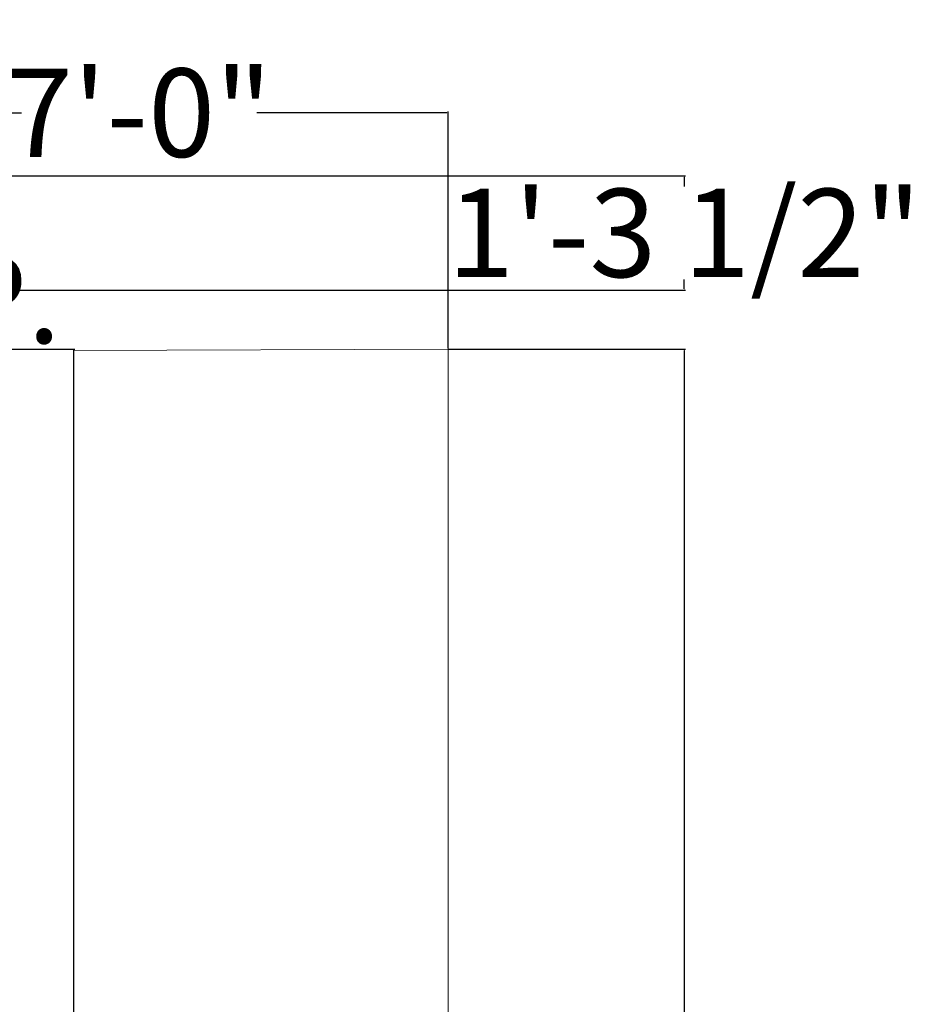
# Model space of a CAD drawing. Units: inches. Extents: x 1063 to 2718, y 423 to 1923.
# Tile 7 of 7: x 1509 to 1630, y 862 to 996. Entities that reach past the tile are written whole.
import ezdxf

# ---------------------------------------------------------------- set-up
doc = ezdxf.new("R2010")
doc.units = ezdxf.units.IN
doc.header["$LTSCALE"] = 6
doc.header["$MEASUREMENT"] = 0
doc.layers.add('A-ANNO-DIMS', color=2, linetype='Continuous', lineweight=18)
doc.layers.add('C-PKNG', color=7, linetype='Continuous', lineweight=18)
doc.styles.get("Standard").update_dxf_attribs({"font": 'arial.ttf'})
doc.dimstyles.get("Standard").update_dxf_attribs({"dimtxt": 12, "dimasz": 0.18, "dimexe": 0.18, "dimexo": 0.0625, "dimgap": 0.09, "dimtad": 0, "dimtih": 1, "dimtoh": 1, "dimdec": 1, "dimzin": 0, "dimdsep": 46, "dimlunit": 3, "dimtxsty": 'Standard', "dimcen": 0.09, "dimadec": 0, "dimazin": 0, "dimtfac": 1, "dimtdec": 1, "dimtofl": 0, "dimtmove": 0, "dimatfit": 3, "dimfxl": 1, "dimtolj": 1, "dimtzin": 0, "dimarcsym": 0})

# ---------------------------------------------------------------- blocks, each defined once
blk = doc.blocks.new('*D3')
at = {"layer": 'A-ANNO-DIMS', "color": 0, "lineweight": -2, "ltscale": 6, "transparency": 16777216}
for p, q in [((1482.99, 951.12), (1516.18, 951.12)), ((1516, 950.94), (1516, 765.34)), ((1516, 567.3), (1516, 752.9)), ((1482.99, 567.12), (1516.18, 567.12))]:
    blk.add_line(p, q, dxfattribs=at)
at = {"layer": 'A-ANNO-DIMS', "color": 0, "ltscale": 6, "transparency": 16777216}
for points in [[(1515.97, 950.94), (1516.03, 950.94), (1516, 951.12)], [(1515.97, 567.3), (1516.03, 567.3), (1516, 567.12)]]:
    blk.add_solid(points, dxfattribs=at)
at = {"layer": 'Defpoints', "color": 0, "ltscale": 6, "transparency": 16777216}
for p in [(1482.93, 951.12), (1516, 951.12), (1482.93, 567.12)]:
    blk.add_point(p, dxfattribs=at)
at = {"layer": 'A-ANNO-DIMS', "color": 0, "ltscale": 6, "transparency": 16777216, "insert": (1516, 759.12), "char_height": 12, "attachment_point": 5}
blk.add_mtext("\\A1;32'", dxfattribs=at)
blk = doc.blocks.new('*D36')
at = {"layer": 'A-ANNO-DIMS', "color": 0, "lineweight": -2, "ltscale": 6, "transparency": 16777216}
for p, q in [((1334.27, 958.87), (1334.27, 957.74)), ((1334.45, 957.92), (1340.83, 957.92)), ((1341.01, 958.87), (1341.01, 957.74)), ((1341.01, 957.92), (1341.19, 957.92))]:
    blk.add_line(p, q, dxfattribs=at)
at = {"layer": 'A-ANNO-DIMS', "color": 0, "ltscale": 6, "transparency": 16777216}
for points in [[(1334.45, 957.95), (1334.45, 957.89), (1334.27, 957.92)], [(1340.83, 957.95), (1340.83, 957.89), (1341.01, 957.92)]]:
    blk.add_solid(points, dxfattribs=at)
at = {"layer": 'Defpoints', "color": 0, "ltscale": 6, "transparency": 16777216}
for p in [(1334.27, 958.93), (1341.01, 958.93), (1341.01, 957.92)]:
    blk.add_point(p, dxfattribs=at)
at = {"layer": 'A-ANNO-DIMS', "color": 0, "ltscale": 6, "transparency": 16777216, "insert": (1429.29, 957.92), "char_height": 12, "attachment_point": 5}
blk.add_mtext('\\A1;BURNER 0\'-6 1/2" TYP.', dxfattribs=at)
blk = doc.blocks.new('*D48')
at = {"layer": 'A-ANNO-DIMS', "color": 0, "lineweight": -2, "ltscale": 6, "transparency": 16777216}
for p, q in [((1482.93, 951.18), (1482.93, 983.4)), ((1483.11, 983.22), (1508.94, 983.22)), ((1566.75, 983.22), (1540.92, 983.22)), ((1566.93, 951.18), (1566.93, 983.4))]:
    blk.add_line(p, q, dxfattribs=at)
at = {"layer": 'A-ANNO-DIMS', "color": 0, "ltscale": 6, "transparency": 16777216}
for points in [[(1483.11, 983.25), (1483.11, 983.19), (1482.93, 983.22)], [(1566.75, 983.25), (1566.75, 983.19), (1566.93, 983.22)]]:
    blk.add_solid(points, dxfattribs=at)
at = {"layer": 'Defpoints', "color": 0, "ltscale": 6, "transparency": 16777216}
for p in [(1566.93, 983.22), (1482.93, 951.12), (1566.93, 951.12)]:
    blk.add_point(p, dxfattribs=at)
at = {"layer": 'A-ANNO-DIMS', "color": 0, "ltscale": 6, "transparency": 16777216, "insert": (1524.93, 983.22), "char_height": 12, "attachment_point": 5}
blk.add_mtext('\\A1;7\'-0"', dxfattribs=at)
blk = doc.blocks.new('*D49')
at = {"layer": 'A-ANNO-DIMS', "color": 0, "lineweight": -2, "ltscale": 6, "transparency": 16777216}
for p, q in [((1566.99, 951.12), (1599.21, 951.12)), ((1599.03, 950.94), (1599.03, 847.34)), ((1599.03, 731.3), (1599.03, 834.9)), ((1566.99, 731.12), (1599.21, 731.12))]:
    blk.add_line(p, q, dxfattribs=at)
at = {"layer": 'A-ANNO-DIMS', "color": 0, "ltscale": 6, "transparency": 16777216}
for points in [[(1599, 950.94), (1599.06, 950.94), (1599.03, 951.12)], [(1599, 731.3), (1599.06, 731.3), (1599.03, 731.12)]]:
    blk.add_solid(points, dxfattribs=at)
at = {"layer": 'Defpoints', "color": 0, "ltscale": 6, "transparency": 16777216}
for p in [(1566.93, 951.12), (1599.03, 951.12), (1566.93, 731.12)]:
    blk.add_point(p, dxfattribs=at)
at = {"layer": 'A-ANNO-DIMS', "color": 0, "ltscale": 6, "transparency": 16777216, "insert": (1599.03, 841.12), "char_height": 12, "attachment_point": 5}
blk.add_mtext('\\A1;18\'-4"', dxfattribs=at)
blk = doc.blocks.new('*D63')
at = {"layer": 'A-ANNO-DIMS', "color": 0, "lineweight": -2, "ltscale": 6, "transparency": 16777216}
for p, q in [((1395.14, 974.67), (1599.21, 974.67)), ((1599.03, 974.49), (1599.03, 973.19)), ((1599.03, 959.29), (1599.03, 960.59)), ((1393.14, 959.11), (1599.21, 959.11))]:
    blk.add_line(p, q, dxfattribs=at)
at = {"layer": 'A-ANNO-DIMS', "color": 0, "ltscale": 6, "transparency": 16777216}
for points in [[(1599, 974.49), (1599.06, 974.49), (1599.03, 974.67)], [(1599, 959.29), (1599.06, 959.29), (1599.03, 959.11)]]:
    blk.add_solid(points, dxfattribs=at)
at = {"layer": 'Defpoints', "color": 0, "ltscale": 6, "transparency": 16777216}
for p in [(1395.08, 974.67), (1393.08, 959.11), (1599.03, 959.11)]:
    blk.add_point(p, dxfattribs=at)
at = {"layer": 'A-ANNO-DIMS', "color": 0, "ltscale": 6, "transparency": 16777216, "insert": (1599.03, 966.89), "char_height": 12, "attachment_point": 5}
blk.add_mtext('\\A1;1\'-3 1/2"', dxfattribs=at)

msp = doc.modelspace()

# ---------------------------------------------------------------- linework, layer by layer
at = {"layer": 'C-PKNG', "ltscale": 6}
for p, q in [((1566.93, 951.12), (1515.97, 950.94)), ((1566.93, 731.12), (1566.93, 951.12))]:
    msp.add_line(p, q, dxfattribs=at)

# ---------------------------------------------------------------- dimensions: what is measured, and where the dimension line sits
at = {"layer": 'A-ANNO-DIMS', "ltscale": 6}
dim = msp.add_linear_dim(base=(1341.01, 957.92), p1=(1334.27, 958.93), p2=(1341.01, 958.93), text='BURNER <> TYP.', dimstyle='Standard', override={"dimdec": 1, "dimlfac": 1, "dimrnd": 0, "dimzin": 1, "dimdsep": 46, "dimlunit": 4, "dimfrac": 2}, dxfattribs=at)
dim.commit()
dim.dimension.update_dxf_attribs({"geometry": '*D36', "text_midpoint": (1429.29, 957.92)})
for base, p1, p2, angle, override, picture, middle in [((1566.93, 983.22), (1482.93, 951.12), (1566.93, 951.12), 0, {"dimdec": 1, "dimlfac": 1, "dimrnd": 0, "dimzin": 1, "dimdsep": 46, "dimlunit": 4, "dimfrac": 2}, '*D48', (1524.93, 983.22)), ((1599.03, 959.11), (1395.08, 974.67), (1393.08, 959.11), 90, {"dimdec": 1, "dimlfac": 1, "dimrnd": 0, "dimzin": 1, "dimdsep": 46, "dimlunit": 4, "dimfrac": 2}, '*D63', (1599.03, 966.89)), ((1516, 951.12), (1482.93, 567.12), (1482.93, 951.12), 90, {"dimclrd": 0, "dimclre": 0, "dimclrt": 0}, '*D3', (1516, 759.12)), ((1599.03, 951.12), (1566.93, 731.12), (1566.93, 951.12), 90, {"dimdec": 1, "dimlfac": 1, "dimrnd": 0, "dimzin": 1, "dimdsep": 46, "dimlunit": 4, "dimfrac": 2}, '*D49', (1599.03, 841.12))]:
    dim = msp.add_linear_dim(base=base, p1=p1, p2=p2, angle=angle, dimstyle='Standard', override=override, dxfattribs=at)
    dim.commit()
    dim.dimension.update_dxf_attribs({"geometry": picture, "text_midpoint": middle})

doc.saveas('drawing.dxf')
